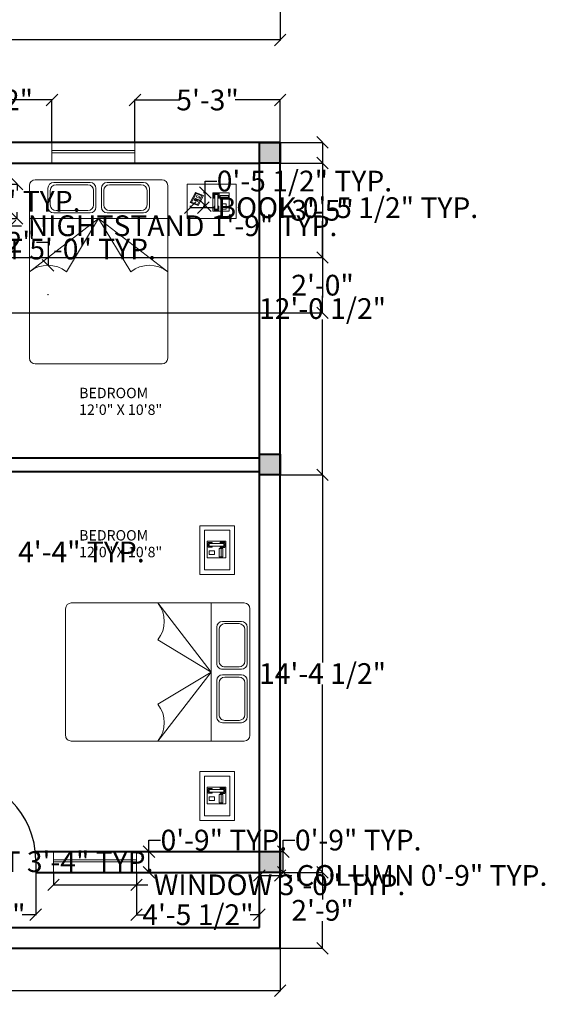
# Model space of a CAD drawing. Units: inches. Extents: x -19 to 1000, y -122 to 1144.
# Tile 3 of 8: x 270 to 498, y -115 to 313. Entities that reach past the tile are written whole.
import ezdxf

# ---------------------------------------------------------------- set-up
doc = ezdxf.new("R2010")
doc.units = ezdxf.units.IN
doc.header["$MEASUREMENT"] = 0
for name, color, linetype, lineweight in [('A-ANNO-DIMS', 191, 'Continuous', 18), ('A-AREA-IDEN', 1, 'Continuous', 18), ('A-COLS', 4, 'Continuous', 40), ('A-COLS-PATT', 220, 'Continuous', 13), ('A-EQPM', 120, 'Continuous', 18), ('A-FURN-PATT', 254, 'Continuous', 13), ('DOORS', 2, 'Continuous', 25), ('FURNITURE', 120, 'Continuous', 18), ('WALLS', 4, 'Continuous', 40), ('WINDOWS', 3, 'Continuous', 18)]:
    doc.layers.add(name, color=color, linetype=linetype, lineweight=lineweight)
doc.styles.get("Standard").update_dxf_attribs({"font": 'arial.ttf'})
doc.dimstyles.get("Standard").update_dxf_attribs({"dimtxt": 9, "dimasz": 5, "dimexe": 0.18, "dimexo": 0.0625, "dimgap": 0.09, "dimtad": 0, "dimtih": 1, "dimtoh": 1, "dimdec": 0, "dimzin": 0, "dimdsep": 46, "dimlunit": 3, "dimtxsty": 'Standard', "dimblk": 'OBLIQUE', "dimcen": 0.09, "dimadec": 0, "dimazin": 0, "dimtfac": 1, "dimtdec": 0, "dimtofl": 0, "dimtmove": 0, "dimatfit": 3, "dimfxl": 1, "dimtolj": 1, "dimtzin": 0, "dimarcsym": 0})

# ---------------------------------------------------------------- blocks, each defined once
blk = doc.blocks.new('Phone - Desk')
for p, q in [((-4.5, -5), (-4.5, 5)), ((-4.5, 5), (4.5, 5)), ((-4, 4.5), (-4, 2)), ((-4, 2), (-3.25, 2)), ((-3.75, 4.5), (-3.75, 2.25)), ((-1.25, 4.5), (-3.75, 4.5)), ((-3.75, 2.25), (-3.25, 2.25)), ((-3.25, 4), (-3.25, -4)), ((-3.25, 4), (-1.75, 4)), ((-1.75, -4), (-1.75, 4)), ((-1.75, 2.25), (-1.25, 2.25)), ((-1.75, 2), (-1, 2)), ((-1.25, 2.25), (-1.25, 4.5)), ((-1, 2), (-1, 4.5)), ((4, 3.5), (-0.5, 3.5)), ((-0.5, 3.5), (-0.5, 1.5)), ((-0.5, 2.5), (4, 2.5)), ((-0.5, 1.5), (4, 1.5)), ((4, 1.5), (4, 3.5)), ((4.5, 5), (4.5, -5)), ((4.5, -5), (-4.5, -5)), ((-3.75, -2.25), (-3.25, -2.25)), ((-3.75, -4.5), (-3.75, -2.25)), ((-1.25, -4.5), (-3.75, -4.5)), ((-3.25, -4), (-1.75, -4)), ((-1.75, -2.25), (-1.25, -2.25)), ((-1.25, -2.25), (-1.25, -4.5)), ((2.75, -1), (0.75, -1)), ((0.75, -1), (0.75, -4)), ((0.75, -4), (2.75, -4)), ((2.75, -4), (2.75, -1))]:
    blk.add_line(p, q)
blk = doc.blocks.new('*U3')
for p, q in [((0, 0), (0, -6)), ((40, 0), (40, -6))]:
    blk.add_line(p, q)
blk.add_lwpolyline([(0, 0), (0, 40), (1.75, 40), (1.75, 0)], close=True)
blk.add_arc((0, 0), 40, 0, 90)
blk = doc.blocks.new('BED-DOUBLE')
for p, q in [((0, 2.5), (0, 77.5)), ((2.5, 80), (57.5, 80)), ((10.5, 78.8), (26.3, 78.8)), ((11.5, 77.8), (25.3, 77.8)), ((33.7, 78.8), (49.5, 78.8)), ((34.7, 77.8), (48.5, 77.8)), ((60, 77.5), (60, 2.5)), ((8, 68.1), (8, 76.3)), ((9, 69.1), (9, 75.3)), ((27.8, 75.3), (27.8, 69.1)), ((28.8, 76.3), (28.8, 68.1)), ((31.2, 68.1), (31.2, 76.3)), ((32.2, 69.1), (32.2, 75.3)), ((51, 75.3), (51, 69.1)), ((52, 76.3), (52, 68.1)), ((10.5, 65.6), (26.3, 65.6)), ((11.5, 66.6), (25.3, 66.6)), ((33.7, 65.6), (49.5, 65.6)), ((34.7, 66.6), (48.5, 66.6)), ((60, 63.2), (0, 63.2)), ((30, 63.2), (0, 40)), ((30, 63.2), (16.04, 40)), ((30, 63.2), (60, 40)), ((30, 63.2), (43.96, 40)), ((57.5, 0), (2.5, 0))]:
    blk.add_line(p, q)
for centre, radius, start, end in [((2.5, 77.5), 2.5, 90, 180), ((10.5, 76.3), 2.5, 90, 180), ((11.5, 75.3), 2.5, 90, 180), ((25.3, 75.3), 2.5, 0, 90), ((26.3, 76.3), 2.5, 0, 90), ((33.7, 76.3), 2.5, 90, 180), ((34.7, 75.3), 2.5, 90, 180), ((48.5, 75.3), 2.5, 0, 90), ((49.5, 76.3), 2.5, 0, 90), ((57.5, 77.5), 2.5, 0, 90), ((11.5, 69.1), 2.5, 180, 270), ((25.3, 69.1), 2.5, 270, 0), ((34.7, 69.1), 2.5, 180, 270), ((48.5, 69.1), 2.5, 270, 0), ((10.5, 68.1), 2.5, 180, 270), ((26.3, 68.1), 2.5, 270, 0), ((33.7, 68.1), 2.5, 180, 270), ((49.5, 68.1), 2.5, 270, 0), ((8.02, 30.16), 12.7, 50.8272, 129.1728), ((51.98, 30.16), 12.7, 50.8272, 129.1728), ((2.5, 2.5), 2.5, 180, 270), ((57.5, 2.5), 2.5, 270, 0)]:
    blk.add_arc(centre, radius, start, end)
blk = doc.blocks.new('TABLE-BEDSIDE')
for points in [[(0, 0), (21.2, 0), (21.2, 14.94), (0, 14.94)], [(2, 2), (19.2, 2), (19.2, 12.94), (2, 12.94)]]:
    blk.add_lwpolyline(points, close=True)
blk = doc.blocks.new('BOOK-PLAN')
for p, q in [((0, 1.37), (2.34, 5.69)), ((2.34, 5.69), (5.74, 4.34)), ((2.6, 5.21), (2.34, 5.69)), ((2.65, 3.83), (2.98, 4.35)), ((2.98, 4.35), (4.3, 3.83)), ((3.43, 0), (5.74, 4.34)), ((0.61, 1.52), (0, 1.37)), ((0, 1.37), (3.43, 0)), ((3.29, 1.76), (1.59, 2.41)), ((3.42, 2.02), (1.72, 2.68)), ((3.6, 2.31), (1.9, 2.97)), ((3.73, 2.58), (2.03, 3.23)), ((2.65, 3.83), (3.97, 3.3)), ((3.97, 3.3), (4.3, 3.83))]:
    blk.add_line(p, q)
blk.add_lwpolyline([(2.6, 5.21), (5.13, 4.2), (3.16, 0.5), (0.61, 1.52)], close=True)
blk = doc.blocks.new('WIN-36-PLAN')
for p, q in [((0, 4.5), (0, 9)), ((0, 9), (0, 0)), ((36, 9), (36, 0)), ((0, 5.5), (36, 5.5)), ((0, 5.5), (36, 5.5)), ((0, 4.5), (36, 4.5))]:
    blk.add_line(p, q)
blk = doc.blocks.new('COLUMN-9X9')
blk.add_lwpolyline([(0, 9), (9, 9), (9, 0), (0, 0)], close=True)
blk = doc.blocks.new('_Oblique')
at = {"color": 0, "linetype": 'ByBlock', "lineweight": -2}
blk.add_line((-0.5, -0.5), (0.5, 0.5), dxfattribs=at)
blk = doc.blocks.new('*D33')
at = {"layer": 'A-ANNO-DIMS', "color": 0, "lineweight": -2, "transparency": 16777216}
for p, q in [((373.64, -57.36), (373.64, -58.82)), ((373.64, -58.64), (382.64, -58.64)), ((382.64, -57.36), (382.64, -58.82)), ((382.64, -58.64), (387.64, -58.64))]:
    blk.add_line(p, q, dxfattribs=at)
at = {"layer": 'Defpoints', "color": 0, "transparency": 16777216}
for p in [(373.64, -57.29), (382.64, -57.29), (382.64, -58.64)]:
    blk.add_point(p, dxfattribs=at)
at = {"layer": 'A-ANNO-DIMS', "color": 0, "lineweight": -2, "transparency": 16777216, "xscale": 5, "yscale": 5, "zscale": 5, "rotation": 180}
blk.add_blockref('_Oblique', (373.64, -58.64), dxfattribs=at)
at = {"layer": 'A-ANNO-DIMS', "color": 0, "lineweight": -2, "transparency": 16777216, "xscale": 5, "yscale": 5, "zscale": 5}
blk.add_blockref('_Oblique', (382.64, -58.64), dxfattribs=at)
at = {"layer": 'A-ANNO-DIMS', "color": 0, "transparency": 16777216, "insert": (444.1, -58.64), "char_height": 9, "attachment_point": 5}
blk.add_mtext('\\A1;COLUMN 0\'-9" TYP.', dxfattribs=at)
blk = doc.blocks.new('*D34')
at = {"layer": 'A-ANNO-DIMS', "color": 0, "lineweight": -2, "transparency": 16777216}
for p, q in [((383.99, -48.29), (383.99, -43.29)), ((383.99, -43.29), (388.99, -43.29)), ((382.7, -48.29), (384.17, -48.29)), ((383.99, -57.29), (383.99, -48.29)), ((382.7, -57.29), (384.17, -57.29))]:
    blk.add_line(p, q, dxfattribs=at)
at = {"layer": 'Defpoints', "color": 0, "transparency": 16777216}
for p in [(382.64, -48.29), (383.99, -48.29), (382.64, -57.29)]:
    blk.add_point(p, dxfattribs=at)
at = {"layer": 'A-ANNO-DIMS', "color": 0, "lineweight": -2, "transparency": 16777216, "xscale": 5, "yscale": 5, "zscale": 5}
for p, rotation in [((383.99, -48.29), 90), ((383.99, -57.29), 270)]:
    blk.add_blockref('_Oblique', p, dxfattribs=dict(at, rotation=rotation))
at = {"layer": 'A-ANNO-DIMS', "color": 0, "transparency": 16777216, "insert": (416.51, -43.29), "char_height": 9, "attachment_point": 5}
blk.add_mtext('\\A1;0\'-9" TYP.', dxfattribs=at)
blk = doc.blocks.new('*D43')
at = {"layer": 'A-ANNO-DIMS', "color": 0, "lineweight": -2, "transparency": 16777216}
for p, q in [((244.17, 226.6), (244.17, 223.31)), ((244.17, 223.49), (265.37, 223.49)), ((265.37, 226.6), (265.37, 223.31)), ((265.37, 223.49), (270.37, 223.49))]:
    blk.add_line(p, q, dxfattribs=at)
at = {"layer": 'Defpoints', "color": 0, "transparency": 16777216}
for p in [(244.17, 226.67), (265.37, 226.67), (265.37, 223.49)]:
    blk.add_point(p, dxfattribs=at)
at = {"layer": 'A-ANNO-DIMS', "color": 0, "lineweight": -2, "transparency": 16777216, "xscale": 5, "yscale": 5, "zscale": 5, "rotation": 180}
blk.add_blockref('_Oblique', (244.17, 223.49), dxfattribs=at)
at = {"layer": 'A-ANNO-DIMS', "color": 0, "lineweight": -2, "transparency": 16777216, "xscale": 5, "yscale": 5, "zscale": 5}
blk.add_blockref('_Oblique', (265.37, 223.49), dxfattribs=at)
at = {"layer": 'A-ANNO-DIMS', "color": 0, "transparency": 16777216, "insert": (340.28, 223.49), "char_height": 9, "attachment_point": 5}
blk.add_mtext('\\A1;NIGHTSTAND 1\'-9" TYP.', dxfattribs=at)
blk = doc.blocks.new('*D44')
at = {"layer": 'A-ANNO-DIMS', "color": 0, "lineweight": -2, "transparency": 16777216}
for p, q in [((265.43, 241.6), (268.73, 241.6)), ((268.55, 241.6), (268.55, 238.82)), ((265.43, 226.67), (268.73, 226.67)), ((268.55, 226.67), (268.55, 229.45))]:
    blk.add_line(p, q, dxfattribs=at)
at = {"layer": 'Defpoints', "color": 0, "transparency": 16777216}
for p in [(265.37, 241.6), (268.55, 241.6), (265.37, 226.67)]:
    blk.add_point(p, dxfattribs=at)
at = {"layer": 'A-ANNO-DIMS', "color": 0, "lineweight": -2, "transparency": 16777216, "xscale": 5, "yscale": 5, "zscale": 5}
for p, rotation in [((268.55, 241.6), 90), ((268.55, 226.67), 270)]:
    blk.add_blockref('_Oblique', p, dxfattribs=dict(at, rotation=rotation))
at = {"layer": 'A-ANNO-DIMS', "color": 0, "transparency": 16777216, "insert": (268.55, 234.13), "char_height": 9, "attachment_point": 5}
blk.add_mtext('\\A1;1\'-3" TYP.', dxfattribs=at)
blk = doc.blocks.new('*D45')
at = {"layer": 'A-ANNO-DIMS', "color": 0, "lineweight": -2, "transparency": 16777216}
for p, q in [((284.29, -57.36), (284.29, -62.87)), ((320.29, -57.36), (320.29, -62.87)), ((284.29, -62.69), (320.29, -62.69)), ((320.29, -62.69), (325.29, -62.69))]:
    blk.add_line(p, q, dxfattribs=at)
at = {"layer": 'Defpoints', "color": 0, "transparency": 16777216}
for p in [(284.29, -57.29), (320.29, -57.29), (320.29, -62.69)]:
    blk.add_point(p, dxfattribs=at)
at = {"layer": 'A-ANNO-DIMS', "color": 0, "lineweight": -2, "transparency": 16777216, "xscale": 5, "yscale": 5, "zscale": 5, "rotation": 180}
blk.add_blockref('_Oblique', (284.29, -62.69), dxfattribs=at)
at = {"layer": 'A-ANNO-DIMS', "color": 0, "lineweight": -2, "transparency": 16777216, "xscale": 5, "yscale": 5, "zscale": 5}
blk.add_blockref('_Oblique', (320.29, -62.69), dxfattribs=at)
at = {"layer": 'A-ANNO-DIMS', "color": 0, "transparency": 16777216, "insert": (382.33, -62.69), "char_height": 9, "attachment_point": 5}
blk.add_mtext('\\A1;WINDOW 3\'-0" TYP.', dxfattribs=at)
blk = doc.blocks.new('*D46')
at = {"layer": 'A-ANNO-DIMS', "color": 0, "lineweight": -2, "transparency": 16777216}
for p, q in [((325.69, -48.29), (325.69, -43.29)), ((325.69, -43.29), (330.69, -43.29)), ((320.36, -48.29), (325.87, -48.29)), ((325.69, -57.29), (325.69, -48.29)), ((320.36, -57.29), (325.87, -57.29))]:
    blk.add_line(p, q, dxfattribs=at)
at = {"layer": 'Defpoints', "color": 0, "transparency": 16777216}
for p in [(320.29, -48.29), (325.69, -48.29), (320.29, -57.29)]:
    blk.add_point(p, dxfattribs=at)
at = {"layer": 'A-ANNO-DIMS', "color": 0, "lineweight": -2, "transparency": 16777216, "xscale": 5, "yscale": 5, "zscale": 5}
for p, rotation in [((325.69, -48.29), 90), ((325.69, -57.29), 270)]:
    blk.add_blockref('_Oblique', p, dxfattribs=dict(at, rotation=rotation))
at = {"layer": 'A-ANNO-DIMS', "color": 0, "transparency": 16777216, "insert": (358.21, -43.29), "char_height": 9, "attachment_point": 5}
blk.add_mtext('\\A1;0\'-9" TYP.', dxfattribs=at)
blk = doc.blocks.new('*D55')
at = {"layer": 'A-ANNO-DIMS', "color": 0, "lineweight": -2, "transparency": 16777216}
for p, q in [((142.9, 222.31), (142.9, 213.19)), ((202.9, 222.31), (202.9, 213.19)), ((142.9, 213.37), (202.9, 213.37)), ((202.9, 213.37), (207.9, 213.37))]:
    blk.add_line(p, q, dxfattribs=at)
at = {"layer": 'Defpoints', "color": 0, "transparency": 16777216}
for p in [(142.9, 222.37), (202.9, 222.37), (202.9, 213.37)]:
    blk.add_point(p, dxfattribs=at)
at = {"layer": 'A-ANNO-DIMS', "color": 0, "lineweight": -2, "transparency": 16777216, "xscale": 5, "yscale": 5, "zscale": 5, "rotation": 180}
blk.add_blockref('_Oblique', (142.9, 213.37), dxfattribs=at)
at = {"layer": 'A-ANNO-DIMS', "color": 0, "lineweight": -2, "transparency": 16777216, "xscale": 5, "yscale": 5, "zscale": 5}
blk.add_blockref('_Oblique', (202.9, 213.37), dxfattribs=at)
at = {"layer": 'A-ANNO-DIMS', "color": 0, "transparency": 16777216, "insert": (270.16, 213.37), "char_height": 9, "attachment_point": 5}
blk.add_mtext('\\A1;LOVESEAT 5\'-0" TYP.', dxfattribs=at)
blk = doc.blocks.new('*D59')
at = {"layer": 'A-ANNO-DIMS', "color": 0, "lineweight": -2, "transparency": 16777216}
for p, q in [((124.63, 89.6), (124.63, 81.68)), ((176.6, 89.6), (176.6, 81.68)), ((124.63, 81.86), (176.6, 81.86)), ((176.6, 81.86), (181.6, 81.86))]:
    blk.add_line(p, q, dxfattribs=at)
at = {"layer": 'Defpoints', "color": 0, "transparency": 16777216}
for p in [(124.63, 89.66), (176.6, 89.66), (176.6, 81.86)]:
    blk.add_point(p, dxfattribs=at)
at = {"layer": 'A-ANNO-DIMS', "color": 0, "lineweight": -2, "transparency": 16777216, "xscale": 5, "yscale": 5, "zscale": 5, "rotation": 180}
blk.add_blockref('_Oblique', (124.63, 81.86), dxfattribs=at)
at = {"layer": 'A-ANNO-DIMS', "color": 0, "lineweight": -2, "transparency": 16777216, "xscale": 5, "yscale": 5, "zscale": 5}
blk.add_blockref('_Oblique', (176.6, 81.86), dxfattribs=at)
at = {"layer": 'A-ANNO-DIMS', "color": 0, "transparency": 16777216, "insert": (254.31, 81.86), "char_height": 9, "attachment_point": 5}
blk.add_mtext('\\A1;DINING TABLE 4\'-4" TYP.', dxfattribs=at)
blk = doc.blocks.new('*D61')
at = {"layer": 'A-ANNO-DIMS', "color": 0, "lineweight": -2, "transparency": 16777216}
for p, q in [((343.57, 232.15), (343.57, 231.17)), ((343.57, 231.35), (349.31, 231.35)), ((349.31, 232.15), (349.31, 231.17)), ((349.31, 231.35), (354.31, 231.35))]:
    blk.add_line(p, q, dxfattribs=at)
at = {"layer": 'Defpoints', "color": 0, "transparency": 16777216}
for p in [(343.57, 232.21), (349.31, 232.21), (349.31, 231.35)]:
    blk.add_point(p, dxfattribs=at)
at = {"layer": 'A-ANNO-DIMS', "color": 0, "lineweight": -2, "transparency": 16777216, "xscale": 5, "yscale": 5, "zscale": 5, "rotation": 180}
blk.add_blockref('_Oblique', (343.57, 231.35), dxfattribs=at)
at = {"layer": 'A-ANNO-DIMS', "color": 0, "lineweight": -2, "transparency": 16777216, "xscale": 5, "yscale": 5, "zscale": 5}
blk.add_blockref('_Oblique', (349.31, 231.35), dxfattribs=at)
at = {"layer": 'A-ANNO-DIMS', "color": 0, "transparency": 16777216, "insert": (412.03, 231.35), "char_height": 9, "attachment_point": 5}
blk.add_mtext('\\A1;BOOK 0\'-5 1/2" TYP.', dxfattribs=at)
blk = doc.blocks.new('*D62')
at = {"layer": 'A-ANNO-DIMS', "color": 0, "lineweight": -2, "transparency": 16777216}
for p, q in [((350.17, 237.91), (350.17, 242.91)), ((350.17, 242.91), (355.17, 242.91)), ((349.37, 237.91), (350.35, 237.91)), ((350.17, 232.21), (350.17, 237.91)), ((349.37, 232.21), (350.35, 232.21))]:
    blk.add_line(p, q, dxfattribs=at)
at = {"layer": 'Defpoints', "color": 0, "transparency": 16777216}
for p in [(349.31, 237.91), (350.17, 237.91), (349.31, 232.21)]:
    blk.add_point(p, dxfattribs=at)
at = {"layer": 'A-ANNO-DIMS', "color": 0, "lineweight": -2, "transparency": 16777216, "xscale": 5, "yscale": 5, "zscale": 5}
for p, rotation in [((350.17, 237.91), 90), ((350.17, 232.21), 270)]:
    blk.add_blockref('_Oblique', p, dxfattribs=dict(at, rotation=rotation))
at = {"layer": 'A-ANNO-DIMS', "color": 0, "transparency": 16777216, "insert": (393.18, 242.91), "char_height": 9, "attachment_point": 5}
blk.add_mtext('\\A1;0\'-5 1/2" TYP.', dxfattribs=at)
blk = doc.blocks.new('*D63')
at = {"layer": 'A-ANNO-DIMS', "color": 0, "lineweight": -2, "transparency": 16777216}
for p, q in [((163.91, -46.76), (163.91, -52.87)), ((203.91, -46.76), (203.91, -52.87)), ((163.91, -52.69), (203.91, -52.69)), ((203.91, -52.69), (208.91, -52.69))]:
    blk.add_line(p, q, dxfattribs=at)
at = {"layer": 'Defpoints', "color": 0, "transparency": 16777216}
for p in [(163.91, -46.69), (203.91, -46.69), (203.91, -52.69)]:
    blk.add_point(p, dxfattribs=at)
at = {"layer": 'A-ANNO-DIMS', "color": 0, "lineweight": -2, "transparency": 16777216, "xscale": 5, "yscale": 5, "zscale": 5, "rotation": 180}
blk.add_blockref('_Oblique', (163.91, -52.69), dxfattribs=at)
at = {"layer": 'A-ANNO-DIMS', "color": 0, "lineweight": -2, "transparency": 16777216, "xscale": 5, "yscale": 5, "zscale": 5}
blk.add_blockref('_Oblique', (203.91, -52.69), dxfattribs=at)
at = {"layer": 'A-ANNO-DIMS', "color": 0, "transparency": 16777216, "insert": (269.24, -52.69), "char_height": 9, "attachment_point": 5}
blk.add_mtext('\\A1;SINK UNIT 3\'-4" TYP.', dxfattribs=at)
blk = doc.blocks.new('*D83')
at = {"layer": 'A-ANNO-DIMS', "color": 0, "lineweight": -2, "transparency": 16777216}
for p, q in [((21.64, -90.36), (21.64, -108.87)), ((382.64, -90.36), (382.64, -108.87)), ((21.64, -108.69), (186.6, -108.69)), ((382.64, -108.69), (217.69, -108.69))]:
    blk.add_line(p, q, dxfattribs=at)
at = {"layer": 'Defpoints', "color": 0, "transparency": 16777216}
for p in [(21.64, -90.29), (382.64, -90.29), (382.64, -108.69)]:
    blk.add_point(p, dxfattribs=at)
at = {"layer": 'A-ANNO-DIMS', "color": 0, "lineweight": -2, "transparency": 16777216, "xscale": 5, "yscale": 5, "zscale": 5, "rotation": 180}
blk.add_blockref('_Oblique', (21.64, -108.69), dxfattribs=at)
at = {"layer": 'A-ANNO-DIMS', "color": 0, "lineweight": -2, "transparency": 16777216, "xscale": 5, "yscale": 5, "zscale": 5}
blk.add_blockref('_Oblique', (382.64, -108.69), dxfattribs=at)
at = {"layer": 'A-ANNO-DIMS', "color": 0, "transparency": 16777216, "insert": (202.14, -108.69), "char_height": 9, "attachment_point": 5}
blk.add_mtext('\\A1;30\'-1"', dxfattribs=at)
blk = doc.blocks.new('*D88')
at = {"layer": 'A-ANNO-DIMS', "color": 0, "lineweight": -2, "transparency": 16777216}
for p, q in [((191.15, 259.77), (191.15, 278.29)), ((191.15, 278.11), (223.64, 278.11)), ((223.64, 250.77), (223.64, 278.29)), ((223.64, 278.11), (228.64, 278.11))]:
    blk.add_line(p, q, dxfattribs=at)
at = {"layer": 'Defpoints', "color": 0, "transparency": 16777216}
for p in [(223.64, 278.11), (191.15, 259.71), (223.64, 250.71)]:
    blk.add_point(p, dxfattribs=at)
at = {"layer": 'A-ANNO-DIMS', "color": 0, "lineweight": -2, "transparency": 16777216, "xscale": 5, "yscale": 5, "zscale": 5, "rotation": 180}
blk.add_blockref('_Oblique', (191.15, 278.11), dxfattribs=at)
at = {"layer": 'A-ANNO-DIMS', "color": 0, "lineweight": -2, "transparency": 16777216, "xscale": 5, "yscale": 5, "zscale": 5}
blk.add_blockref('_Oblique', (223.64, 278.11), dxfattribs=at)
at = {"layer": 'A-ANNO-DIMS', "color": 0, "transparency": 16777216, "insert": (251.26, 278.11), "char_height": 9, "attachment_point": 5}
blk.add_mtext('\\A1;2\'-8 1/2"', dxfattribs=at)
blk = doc.blocks.new('*D89')
at = {"layer": 'A-ANNO-DIMS', "color": 0, "lineweight": -2, "transparency": 16777216}
for p, q in [((223.64, 250.77), (223.64, 278.29)), ((223.64, 278.11), (241.59, 278.11)), ((283.63, 278.11), (265.69, 278.11)), ((283.63, 259.77), (283.63, 278.29))]:
    blk.add_line(p, q, dxfattribs=at)
at = {"layer": 'Defpoints', "color": 0, "transparency": 16777216}
for p in [(283.63, 278.11), (283.63, 259.71), (223.64, 250.71)]:
    blk.add_point(p, dxfattribs=at)
at = {"layer": 'A-ANNO-DIMS', "color": 0, "lineweight": -2, "transparency": 16777216, "xscale": 5, "yscale": 5, "zscale": 5, "rotation": 180}
blk.add_blockref('_Oblique', (223.64, 278.11), dxfattribs=at)
at = {"layer": 'A-ANNO-DIMS', "color": 0, "lineweight": -2, "transparency": 16777216, "xscale": 5, "yscale": 5, "zscale": 5}
blk.add_blockref('_Oblique', (283.63, 278.11), dxfattribs=at)
at = {"layer": 'A-ANNO-DIMS', "color": 0, "transparency": 16777216, "insert": (253.64, 278.11), "char_height": 9, "attachment_point": 5}
blk.add_mtext('\\A1;5\'-0"', dxfattribs=at)
blk = doc.blocks.new('*D90')
at = {"layer": 'A-ANNO-DIMS', "color": 0, "lineweight": -2, "transparency": 16777216}
for p, q in [((319.63, 259.77), (319.63, 278.29)), ((319.63, 278.11), (339.09, 278.11)), ((382.64, 278.11), (363.19, 278.11)), ((382.64, 259.77), (382.64, 278.29))]:
    blk.add_line(p, q, dxfattribs=at)
at = {"layer": 'Defpoints', "color": 0, "transparency": 16777216}
for p in [(382.64, 278.11), (319.63, 259.71), (382.64, 259.71)]:
    blk.add_point(p, dxfattribs=at)
at = {"layer": 'A-ANNO-DIMS', "color": 0, "lineweight": -2, "transparency": 16777216, "xscale": 5, "yscale": 5, "zscale": 5, "rotation": 180}
blk.add_blockref('_Oblique', (319.63, 278.11), dxfattribs=at)
at = {"layer": 'A-ANNO-DIMS', "color": 0, "lineweight": -2, "transparency": 16777216, "xscale": 5, "yscale": 5, "zscale": 5}
blk.add_blockref('_Oblique', (382.64, 278.11), dxfattribs=at)
at = {"layer": 'A-ANNO-DIMS', "color": 0, "transparency": 16777216, "insert": (351.14, 278.11), "char_height": 9, "attachment_point": 5}
blk.add_mtext('\\A1;5\'-3"', dxfattribs=at)
blk = doc.blocks.new('*D91')
at = {"layer": 'A-ANNO-DIMS', "color": 0, "lineweight": -2, "transparency": 16777216}
for p, q in [((382.7, -57.29), (401.22, -57.29)), ((401.04, -57.29), (401.04, -69.11)), ((401.04, -90.29), (401.04, -78.48)), ((382.7, -90.29), (401.22, -90.29))]:
    blk.add_line(p, q, dxfattribs=at)
at = {"layer": 'Defpoints', "color": 0, "transparency": 16777216}
for p in [(382.64, -57.29), (401.04, -57.29), (382.64, -90.29)]:
    blk.add_point(p, dxfattribs=at)
at = {"layer": 'A-ANNO-DIMS', "color": 0, "lineweight": -2, "transparency": 16777216, "xscale": 5, "yscale": 5, "zscale": 5}
for p, rotation in [((401.04, -57.29), 90), ((401.04, -90.29), 270)]:
    blk.add_blockref('_Oblique', p, dxfattribs=dict(at, rotation=rotation))
at = {"layer": 'A-ANNO-DIMS', "color": 0, "transparency": 16777216, "insert": (401.04, -73.79), "char_height": 9, "attachment_point": 5}
blk.add_mtext('\\A1;2\'-9"', dxfattribs=at)
blk = doc.blocks.new('*D92')
at = {"layer": 'A-ANNO-DIMS', "color": 0, "lineweight": -2, "transparency": 16777216}
for p, q in [((382.7, 115.35), (401.22, 115.35)), ((401.04, 115.35), (401.04, 33.77)), ((401.04, -57.29), (401.04, 24.29)), ((382.7, -57.29), (401.22, -57.29))]:
    blk.add_line(p, q, dxfattribs=at)
at = {"layer": 'Defpoints', "color": 0, "transparency": 16777216}
for p in [(382.64, 115.35), (401.04, 115.35), (382.64, -57.29)]:
    blk.add_point(p, dxfattribs=at)
at = {"layer": 'A-ANNO-DIMS', "color": 0, "lineweight": -2, "transparency": 16777216, "xscale": 5, "yscale": 5, "zscale": 5}
for p, rotation in [((401.04, 115.35), 90), ((401.04, -57.29), 270)]:
    blk.add_blockref('_Oblique', p, dxfattribs=dict(at, rotation=rotation))
at = {"layer": 'A-ANNO-DIMS', "color": 0, "transparency": 16777216, "insert": (401.04, 29.03), "char_height": 9, "attachment_point": 5}
blk.add_mtext('\\A1;14\'-4 1/2"', dxfattribs=at)
blk = doc.blocks.new('*D93')
at = {"layer": 'A-ANNO-DIMS', "color": 0, "lineweight": -2, "transparency": 16777216}
for p, q in [((382.7, 259.71), (401.22, 259.71)), ((401.04, 259.71), (401.04, 192.27)), ((401.04, 115.35), (401.04, 182.79)), ((382.7, 115.35), (401.22, 115.35))]:
    blk.add_line(p, q, dxfattribs=at)
at = {"layer": 'Defpoints', "color": 0, "transparency": 16777216}
for p in [(382.64, 259.71), (401.04, 259.71), (382.64, 115.35)]:
    blk.add_point(p, dxfattribs=at)
at = {"layer": 'A-ANNO-DIMS', "color": 0, "lineweight": -2, "transparency": 16777216, "xscale": 5, "yscale": 5, "zscale": 5}
for p, rotation in [((401.04, 259.71), 90), ((401.04, 115.35), 270)]:
    blk.add_blockref('_Oblique', p, dxfattribs=dict(at, rotation=rotation))
at = {"layer": 'A-ANNO-DIMS', "color": 0, "transparency": 16777216, "insert": (401.04, 187.53), "char_height": 9, "attachment_point": 5}
blk.add_mtext('\\A1;12\'-0 1/2"', dxfattribs=at)
blk = doc.blocks.new('*D94')
at = {"layer": 'A-ANNO-DIMS', "color": 0, "lineweight": -2, "transparency": 16777216}
for p, q in [((240.57, -57.36), (240.57, -75.87)), ((276.57, -57.36), (276.57, -75.87)), ((240.57, -75.69), (246.52, -75.69)), ((276.57, -75.69), (270.62, -75.69))]:
    blk.add_line(p, q, dxfattribs=at)
at = {"layer": 'Defpoints', "color": 0, "transparency": 16777216}
for p in [(240.57, -57.29), (276.57, -57.29), (240.57, -75.69)]:
    blk.add_point(p, dxfattribs=at)
at = {"layer": 'A-ANNO-DIMS', "color": 0, "lineweight": -2, "transparency": 16777216, "xscale": 5, "yscale": 5, "zscale": 5, "rotation": 180}
blk.add_blockref('_Oblique', (240.57, -75.69), dxfattribs=at)
at = {"layer": 'A-ANNO-DIMS', "color": 0, "lineweight": -2, "transparency": 16777216, "xscale": 5, "yscale": 5, "zscale": 5}
blk.add_blockref('_Oblique', (276.57, -75.69), dxfattribs=at)
at = {"layer": 'A-ANNO-DIMS', "color": 0, "transparency": 16777216, "insert": (258.57, -75.69), "char_height": 9, "attachment_point": 5}
blk.add_mtext('\\A1;3\'-0"', dxfattribs=at)
blk = doc.blocks.new('*D95')
at = {"layer": 'A-ANNO-DIMS', "color": 0, "lineweight": -2, "transparency": 16777216}
for p, q in [((320.29, -57.36), (320.29, -75.87)), ((373.64, -57.36), (373.64, -75.87)), ((320.29, -75.69), (324.25, -75.69)), ((373.64, -75.69), (369.69, -75.69))]:
    blk.add_line(p, q, dxfattribs=at)
at = {"layer": 'Defpoints', "color": 0, "transparency": 16777216}
for p in [(320.29, -57.29), (373.64, -57.29), (320.29, -75.69)]:
    blk.add_point(p, dxfattribs=at)
at = {"layer": 'A-ANNO-DIMS', "color": 0, "lineweight": -2, "transparency": 16777216, "xscale": 5, "yscale": 5, "zscale": 5}
for p, rotation in [((320.29, -75.69), 179.9999999999999), ((373.64, -75.69), 359.9999999999999)]:
    blk.add_blockref('_Oblique', p, dxfattribs=dict(at, rotation=rotation))
at = {"layer": 'A-ANNO-DIMS', "color": 0, "transparency": 16777216, "insert": (346.97, -75.69), "char_height": 9, "attachment_point": 5}
blk.add_mtext('\\A1;4\'-5 1/2"', dxfattribs=at)
blk = doc.blocks.new('*D97')
at = {"layer": 'A-ANNO-DIMS', "color": 0, "lineweight": -2, "transparency": 16777216}
for p, q in [((111.7, 209.69), (401.22, 209.69)), ((401.04, 209.69), (401.04, 202.37)), ((401.04, 185.69), (401.04, 193)), ((111.7, 185.69), (401.22, 185.69))]:
    blk.add_line(p, q, dxfattribs=at)
at = {"layer": 'Defpoints', "color": 0, "transparency": 16777216}
for p in [(111.64, 209.69), (401.04, 209.69), (111.64, 185.69)]:
    blk.add_point(p, dxfattribs=at)
at = {"layer": 'A-ANNO-DIMS', "color": 0, "lineweight": -2, "transparency": 16777216, "xscale": 5, "yscale": 5, "zscale": 5}
for p, rotation in [((401.04, 209.69), 90), ((401.04, 185.69), 270)]:
    blk.add_blockref('_Oblique', p, dxfattribs=dict(at, rotation=rotation))
at = {"layer": 'A-ANNO-DIMS', "color": 0, "transparency": 16777216, "insert": (401.04, 197.69), "char_height": 9, "attachment_point": 5}
blk.add_mtext('\\A1;2\'-0"', dxfattribs=at)
blk = doc.blocks.new('*D99')
at = {"layer": 'A-ANNO-DIMS', "color": 0, "lineweight": -2, "transparency": 16777216}
for p, q in [((105.7, 250.71), (401.22, 250.71)), ((401.04, 250.71), (401.04, 234.89)), ((401.04, 209.69), (401.04, 225.51)), ((111.7, 209.69), (401.22, 209.69))]:
    blk.add_line(p, q, dxfattribs=at)
at = {"layer": 'Defpoints', "color": 0, "transparency": 16777216}
for p in [(105.64, 250.71), (401.04, 250.71), (111.64, 209.69)]:
    blk.add_point(p, dxfattribs=at)
at = {"layer": 'A-ANNO-DIMS', "color": 0, "lineweight": -2, "transparency": 16777216, "xscale": 5, "yscale": 5, "zscale": 5}
for p, rotation in [((401.04, 250.71), 90), ((401.04, 209.69), 270)]:
    blk.add_blockref('_Oblique', p, dxfattribs=dict(at, rotation=rotation))
at = {"layer": 'A-ANNO-DIMS', "color": 0, "transparency": 16777216, "insert": (401.04, 230.2), "char_height": 9, "attachment_point": 5}
blk.add_mtext('\\A1;3\'-5"', dxfattribs=at)
blk = doc.blocks.new('*D111')
at = {"layer": 'A-ANNO-DIMS', "color": 0, "lineweight": -2, "transparency": 16777216}
for p, q in [((21.64, 328.07), (21.64, 304)), ((382.64, 328.07), (382.64, 304)), ((21.64, 304.18), (186.6, 304.18)), ((382.64, 304.18), (217.69, 304.18))]:
    blk.add_line(p, q, dxfattribs=at)
at = {"layer": 'Defpoints', "color": 0, "transparency": 16777216}
for p in [(21.64, 328.13), (382.64, 328.13), (21.64, 304.18)]:
    blk.add_point(p, dxfattribs=at)
at = {"layer": 'A-ANNO-DIMS', "color": 0, "lineweight": -2, "transparency": 16777216, "xscale": 5, "yscale": 5, "zscale": 5, "rotation": 180}
blk.add_blockref('_Oblique', (21.64, 304.18), dxfattribs=at)
at = {"layer": 'A-ANNO-DIMS', "color": 0, "lineweight": -2, "transparency": 16777216, "xscale": 5, "yscale": 5, "zscale": 5}
blk.add_blockref('_Oblique', (382.64, 304.18), dxfattribs=at)
at = {"layer": 'A-ANNO-DIMS', "color": 0, "transparency": 16777216, "insert": (202.14, 304.18), "char_height": 9, "attachment_point": 5}
blk.add_mtext('\\A1;30\'-1"', dxfattribs=at)
blk = doc.blocks.new('*D148')
at = {"layer": 'A-ANNO-DIMS', "color": 0, "lineweight": -2, "transparency": 16777216}
for p, q in [((276.9, 216.33), (281.9, 216.33)), ((281.9, 216.33), (281.9, 206.33)), ((281.81, 193.63), (281.99, 193.63)), ((281.9, 193.54), (281.9, 193.72))]:
    blk.add_line(p, q, dxfattribs=at)
at = {"layer": 'Defpoints', "color": 0, "transparency": 16777216}
for p in [(281.9, 206.33), (281.9, 193.63)]:
    blk.add_point(p, dxfattribs=at)
at = {"layer": 'A-ANNO-DIMS', "color": 0, "lineweight": -2, "transparency": 16777216, "xscale": 5, "yscale": 5, "zscale": 5, "rotation": 270.0006769551681}
blk.add_blockref('_Oblique', (281.9, 206.33), dxfattribs=at)
at = {"layer": 'A-ANNO-DIMS', "color": 0, "transparency": 16777216, "insert": (240.2, 216.33), "char_height": 9, "attachment_point": 5}
blk.add_mtext('\\A1;4X R1\'-0 1/2"', dxfattribs=at)

msp = doc.modelspace()

# ---------------------------------------------------------------- hatches: boundary and pattern name
at = {"layer": 'A-COLS-PATT'}
h = msp.add_hatch(color=256, dxfattribs=at)
h.dxf.hatch_style = 1
h.paths.add_polyline_path([(30.64, 259.71), (21.64, 259.71), (21.64, 250.71), (30.64, 250.71)])
h.paths.add_polyline_path([(113.34, 259.71), (104.34, 259.71), (104.34, 250.71), (113.34, 250.71)])
h.paths.add_polyline_path([(231.33, 259.71), (222.33, 259.71), (222.33, 250.71), (223.64, 250.71), (231.33, 250.71)])
h.paths.add_polyline_path([(382.64, 259.71), (373.64, 259.71), (373.64, 250.71), (382.64, 250.71)])
h.paths.add_polyline_path([(382.64, 124.35), (373.64, 124.35), (373.64, 115.35), (382.64, 115.35)])
h.paths.add_polyline_path([(382.64, -48.29), (373.64, -48.29), (373.64, -57.29), (382.64, -57.29)])
h.paths.add_polyline_path([(111.64, -48.29), (105.64, -48.29), (105.64, -57.29), (111.64, -57.29)])
h.paths.add_polyline_path([(30.64, -48.11), (21.64, -48.11), (21.64, -57.11), (30.64, -57.11)])
h.paths.add_polyline_path([(30.64, 124.5), (21.64, 124.5), (21.64, 115.5), (30.64, 115.5)])
h.paths.add_polyline_path([(111.64, 122.71), (105.64, 122.71), (105.64, 116.71), (111.64, 116.71)])
h.paths.add_polyline_path([(229.64, 122.71), (223.64, 122.71), (223.64, 116.71), (229.64, 116.71)])
h.paths.add_polyline_path([(229.64, -48.29), (223.64, -48.29), (223.64, -57.29), (229.64, -57.29)])
at = {"layer": 'A-FURN-PATT'}
h = msp.add_hatch(color=256, dxfattribs=at)
h.dxf.hatch_style = 1
h.paths.add_polyline_path([(346.17, 237.43), (345.91, 237.91), (343.57, 233.58), (344.18, 233.74)])
h.paths.add_polyline_path([(349.31, 236.55), (345.91, 237.91), (346.17, 237.43), (348.7, 236.42), (346.73, 232.72), (344.18, 233.74), (343.57, 233.58), (347, 232.21)])

# ---------------------------------------------------------------- linework, layer by layer
at = {"layer": 'FURNITURE'}
msp.add_lwpolyline([(342.31, 226.67), (363.51, 226.67), (363.51, 241.6), (342.31, 241.6)], close=True, dxfattribs=at)
at = {"layer": 'WALLS'}
for p, q in [((382.64, 259.71), (21.64, 259.71)), ((382.64, -90.29), (382.64, 259.71)), ((229.64, 250.71), (373.64, 250.71)), ((373.64, 122.71), (373.64, 250.71)), ((229.64, 122.71), (373.64, 122.71)), ((229.64, 116.71), (373.64, 116.71)), ((373.64, -48.29), (373.64, 116.71)), ((276.39, -48.29), (373.64, -48.29)), ((276.57, -57.29), (373.64, -57.29)), ((373.64, -81.29), (373.64, -57.29)), ((223.64, -81.29), (373.64, -81.29)), ((223.64, -90.29), (382.64, -90.29))]:
    msp.add_line(p, q, dxfattribs=at)

# ---------------------------------------------------------------- block references
at = {"layer": 'A-COLS'}
for p in [(373.64, 250.71), (373.64, 115.35), (373.64, -57.3)]:
    msp.add_blockref('COLUMN-9X9', p, dxfattribs=at)
at = {"layer": 'A-EQPM', "xscale": 0.8015722193121366, "yscale": 0.8015722193121366, "zscale": 0.8015722193121366}
msp.add_blockref('Phone - Desk', (356.97, 233.85), dxfattribs=at)
at = {"layer": 'A-EQPM', "xscale": 0.8015722193121366, "yscale": 0.8015722193121366, "zscale": 0.8015722193121366, "rotation": 270}
for p in [(355, 82.95), (355, -23.87)]:
    msp.add_blockref('Phone - Desk', p, dxfattribs=at)
at = {"layer": 'DOORS', "xscale": 0.9, "yscale": 0.9, "zscale": 0.9}
msp.add_blockref('*U3', (240.57, -51.89), dxfattribs=at)
at = {"layer": 'FURNITURE'}
for name, p in [('BED-DOUBLE', (273.88, 163.47)), ('BOOK-PLAN', (343.57, 232.22))]:
    msp.add_blockref(name, p, dxfattribs=at)
for name, p, rotation in [('TABLE-BEDSIDE', (347.82, 93.25), 269.9999999999999), ('BED-DOUBLE', (289.52, 59.7), 270.0000000000002), ('TABLE-BEDSIDE', (347.82, -13.57), 269.9999999999999)]:
    msp.add_blockref(name, p, dxfattribs=dict(at, rotation=rotation))
at = {"layer": 'WINDOWS'}
for p in [(283.63, 250.71), (284.29, -57.3)]:
    msp.add_blockref('WIN-36-PLAN', p, dxfattribs=at)

# ---------------------------------------------------------------- texts
at = {"layer": 'A-AREA-IDEN'}
for s, height, p in [('BEDROOM', 4.516, (295.4, 148.61)), ('12\'0" X 10\'8"', 4.5155, (295.4, 141.36)), ('BEDROOM', 4.516, (295.4, 86.8)), ('12\'0" X 10\'8"', 4.5155, (295.4, 79.54))]:
    msp.add_text(s, height=height, dxfattribs=at).set_placement(p)

# ---------------------------------------------------------------- dimensions: what is measured, and where the dimension line sits
at = {"layer": 'A-ANNO-DIMS'}
for base, p1, p2, angle, picture, middle in [((21.64, 304.18), (382.64, 328.13), (21.64, 328.13), 180, '*D111', (202.14, 304.18)), ((401.04, 259.71), (382.64, 115.35), (382.64, 259.71), 90, '*D93', (401.04, 187.53)), ((401.04, 250.71), (111.64, 209.69), (105.64, 250.71), 90, '*D99', (401.04, 230.2)), ((401.04, 209.69), (111.64, 185.69), (111.64, 209.69), 90, '*D97', (401.04, 197.69)), ((401.04, 115.35), (382.64, -57.29), (382.64, 115.35), 90, '*D92', (401.04, 29.03)), ((401.04, -57.29), (382.64, -90.29), (382.64, -57.29), 90, '*D91', (401.04, -73.79)), ((240.57, -75.69), (276.57, -57.29), (240.57, -57.29), 180, '*D94', (258.57, -75.69)), ((320.293, -75.6945), (373.6418, -57.2945), (320.293, -57.2945), 180, '*D95', (346.9674, -75.6945))]:
    dim = msp.add_linear_dim(base=base, p1=p1, p2=p2, angle=angle, dimstyle='Standard', override={"dimdec": 1, "dimlfac": 1, "dimrnd": 0, "dimzin": 1, "dimdsep": 46, "dimlunit": 4, "dimfrac": 2}, dxfattribs=at)
    dim.commit()
    dim.dimension.update_dxf_attribs({"geometry": picture, "text_midpoint": middle})
for base, p1, p2, picture, middle in [((223.64, 278.11), (191.15, 259.71), (223.64, 250.71), '*D88', (251.26, 278.11)), ((283.63, 278.11), (223.64, 250.71), (283.63, 259.71), '*D89', (253.64, 278.11)), ((382.64, 278.11), (319.63, 259.71), (382.64, 259.71), '*D90', (351.14, 278.11)), ((382.64, -108.69), (21.64, -90.29), (382.64, -90.29), '*D83', (202.14, -108.69))]:
    dim = msp.add_linear_dim(base=base, p1=p1, p2=p2, dimstyle='Standard', override={"dimdec": 1, "dimlfac": 1, "dimrnd": 0, "dimzin": 1, "dimdsep": 46, "dimlunit": 4, "dimfrac": 2}, dxfattribs=at)
    dim.commit()
    dim.dimension.update_dxf_attribs({"geometry": picture, "text_midpoint": middle})
for base, p1, p2, picture, middle in [((350.17, 237.91), (349.31, 232.21), (349.31, 237.91), '*D62', (393.18, 242.91)), ((268.55, 241.6), (265.37, 226.67), (265.37, 241.6), '*D44', (268.55, 234.13)), ((325.69, -48.29), (320.29, -57.29), (320.29, -48.29), '*D46', (358.21, -43.29)), ((383.99, -48.29), (382.64, -57.29), (382.64, -48.29), '*D34', (416.51, -43.29))]:
    dim = msp.add_linear_dim(base=base, p1=p1, p2=p2, angle=90, text='<> TYP.', dimstyle='Standard', override={"dimdec": 1, "dimlfac": 1, "dimrnd": 0, "dimzin": 1, "dimdsep": 46, "dimlunit": 4, "dimfrac": 2}, dxfattribs=at)
    dim.commit()
    dim.dimension.update_dxf_attribs({"geometry": picture, "text_midpoint": middle})
for base, p1, p2, text, picture, middle in [((349.31, 231.35), (343.57, 232.21), (349.31, 232.21), 'BOOK <> TYP.', '*D61', (412.03, 231.35)), ((265.37, 223.49), (244.17, 226.67), (265.37, 226.67), 'NIGHTSTAND <> TYP.', '*D43', (340.28, 223.49)), ((202.9, 213.37), (142.9, 222.37), (202.9, 222.37), 'LOVESEAT <> TYP.', '*D55', (270.16, 213.37)), ((176.6, 81.86), (124.63, 89.66), (176.6, 89.66), 'DINING TABLE <> TYP.', '*D59', (254.31, 81.86)), ((203.91, -52.69), (163.91, -46.69), (203.91, -46.69), 'SINK UNIT <> TYP.', '*D63', (269.24, -52.69)), ((382.64, -58.64), (373.64, -57.29), (382.64, -57.29), 'COLUMN <> TYP.', '*D33', (444.1, -58.64)), ((320.29, -62.69), (284.29, -57.29), (320.29, -57.29), 'WINDOW <> TYP.', '*D45', (382.33, -62.69))]:
    dim = msp.add_linear_dim(base=base, p1=p1, p2=p2, text=text, dimstyle='Standard', override={"dimdec": 1, "dimlfac": 1, "dimrnd": 0, "dimzin": 1, "dimdsep": 46, "dimlunit": 4, "dimfrac": 2}, dxfattribs=at)
    dim.commit()
    dim.dimension.update_dxf_attribs({"geometry": picture, "text_midpoint": middle})
dim = msp.add_radius_dim(center=(281.9, 193.63), mpoint=(281.9, 206.33), text='4X <>', dimstyle='Standard', override={"dimdec": 1, "dimlfac": 1, "dimrnd": 0, "dimzin": 1, "dimdsep": 46, "dimlunit": 4, "dimfrac": 2}, dxfattribs=at)
dim.commit()
dim.dimension.update_dxf_attribs({"geometry": '*D148', "text_midpoint": (240.2, 216.33)})

doc.saveas('drawing.dxf')
